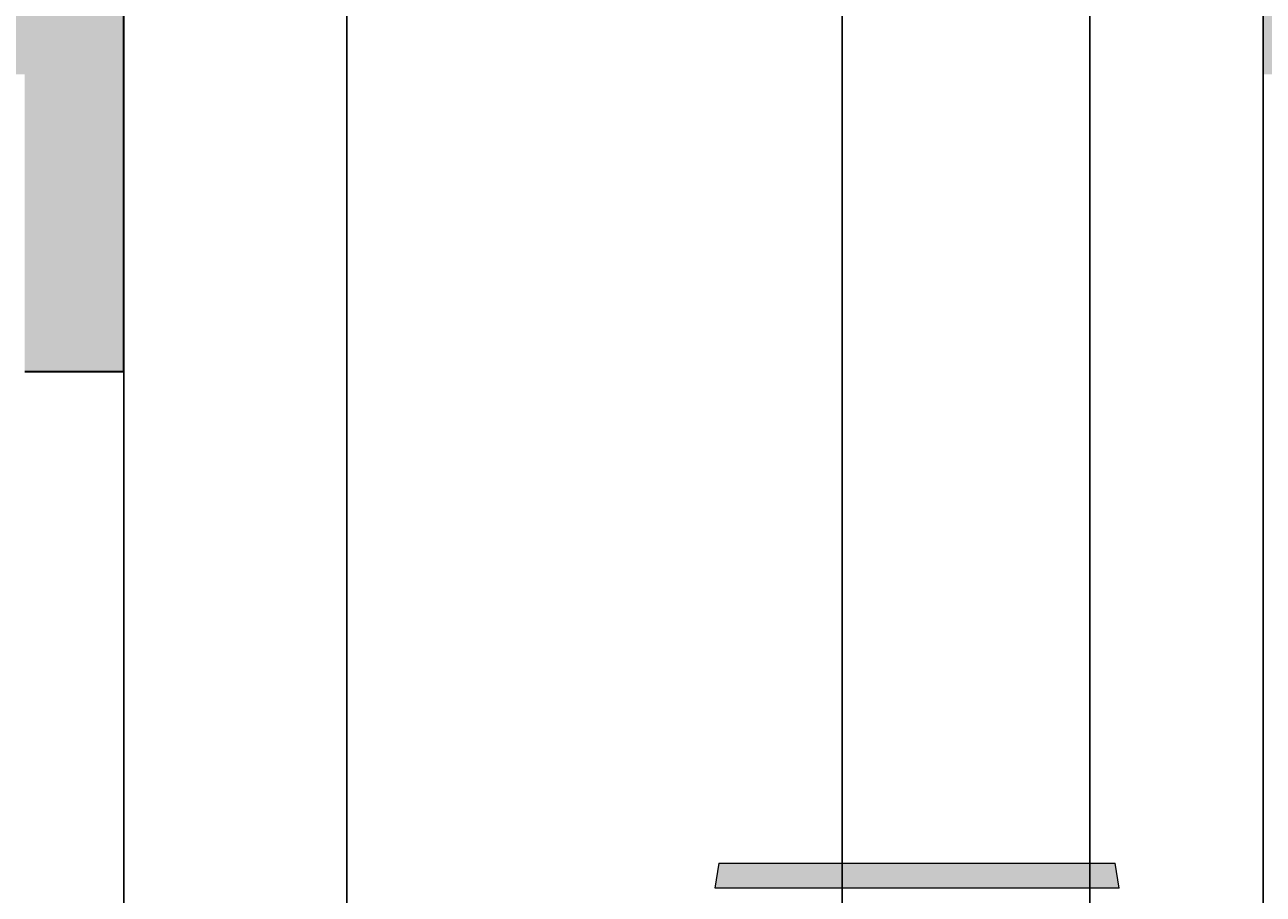
# Model space of a CAD drawing. Units: inches. Extents: x 1567 to 1964, y 1813 to 2447.
# Tile 18 of 28: x 1738 to 1788, y 2226 to 2261. Entities that reach past the tile are written whole.
import ezdxf

# ---------------------------------------------------------------- set-up
doc = ezdxf.new("R2010")
doc.units = ezdxf.units.IN
for name, color, linetype, lineweight in [('A-ANNO-DIMS', 2, 'Continuous', 18), ('A-FURN', 8, 'Continuous', 18), ('A-WALL', 7, 'Continuous', 35)]:
    doc.layers.add(name, color=color, linetype=linetype, lineweight=lineweight)
doc.layers.add('A-FURN-PATT', color=252, linetype='Continuous', lineweight=13, true_color=0x939598)
doc.layers.add('A-WALL-PATT', color=251, linetype='Continuous', lineweight=13, true_color=0x636466)
doc.styles.get("Standard").update_dxf_attribs({"font": 'arial.ttf'})
doc.dimstyles.get("Standard").update_dxf_attribs({"dimtxt": 0.18, "dimasz": 0.18, "dimexe": 0.18, "dimexo": 0.0625, "dimgap": 0.09, "dimtad": 0, "dimtih": 1, "dimtoh": 1, "dimdec": 4, "dimzin": 0, "dimdsep": 46, "dimtxsty": 'Standard', "dimcen": 0.09, "dimadec": 0, "dimazin": 0, "dimtfac": 1, "dimtdec": 4, "dimtofl": 0, "dimtmove": 0, "dimatfit": 3, "dimfxl": 1, "dimtolj": 1, "dimtzin": 0, "dimarcsym": 0})

# ---------------------------------------------------------------- blocks, each defined once
blk = doc.blocks.new('Dining Set - 36 x 72 in.')
for p, q in [((-22, 27.5), (-22.1562, 26.50042)), ((-22, 27.5), (-6, 27.5)), ((-5.8437, 26.49966), (-6, 27.5)), ((-5.8416, 26.5), (-22.1534, 26.5))]:
    blk.add_line(p, q)
blk = doc.blocks.new('*D47')
at = {"layer": 'A-ANNO-DIMS', "color": 0, "lineweight": -2, "transparency": 16777216}
for p, q in [((1742.43, 2331.227), (1742.43, 1813.46)), ((1788.43, 2331.227), (1788.43, 1813.46)), ((1742.61, 1813.64), (1765.207, 1813.64)), ((1788.25, 1813.64), (1765.652, 1813.64))]:
    blk.add_line(p, q, dxfattribs=at)
at = {"layer": 'A-ANNO-DIMS', "color": 0, "transparency": 16777216}
for points in [[(1742.61, 1813.67), (1742.61, 1813.61), (1742.43, 1813.64)], [(1788.25, 1813.67), (1788.25, 1813.61), (1788.43, 1813.64)]]:
    blk.add_solid(points, dxfattribs=at)
at = {"layer": 'Defpoints', "color": 0, "transparency": 16777216}
for p in [(1742.43, 2331.29), (1788.43, 2331.29), (1788.43, 1813.64)]:
    blk.add_point(p, dxfattribs=at)
at = {"layer": 'A-ANNO-DIMS', "color": 0, "transparency": 16777216, "insert": (1765.43, 1813.64), "char_height": 0.18, "attachment_point": 5}
blk.add_mtext('\\A1;46', dxfattribs=at)
blk = doc.blocks.new('*D54')
at = {"layer": 'A-ANNO-DIMS', "color": 0, "lineweight": -2, "transparency": 16777216}
for p, q in [((1711.43, 1964.352), (1711.43, 2447.12)), ((1795.43, 1964.352), (1795.43, 2447.12)), ((1711.61, 2446.94), (1753.211, 2446.94)), ((1795.25, 2446.94), (1753.648, 2446.94))]:
    blk.add_line(p, q, dxfattribs=at)
at = {"layer": 'A-ANNO-DIMS', "color": 0, "transparency": 16777216}
for points in [[(1711.61, 2446.97), (1711.61, 2446.91), (1711.43, 2446.94)], [(1795.25, 2446.97), (1795.25, 2446.91), (1795.43, 2446.94)]]:
    blk.add_solid(points, dxfattribs=at)
at = {"layer": 'Defpoints', "color": 0, "transparency": 16777216}
for p in [(1795.43, 2446.94), (1711.43, 1964.29), (1795.43, 1964.29)]:
    blk.add_point(p, dxfattribs=at)
at = {"layer": 'A-ANNO-DIMS', "color": 0, "transparency": 16777216, "insert": (1753.43, 2446.94), "char_height": 0.18, "attachment_point": 5}
blk.add_mtext('\\A1;84', dxfattribs=at)
blk = doc.blocks.new('*D58')
at = {"layer": 'A-ANNO-DIMS', "color": 0, "lineweight": -2, "transparency": 16777216}
for p, q in [((1742.43, 2127.352), (1742.43, 2447.12)), ((1751.43, 2127.352), (1751.43, 2447.12)), ((1742.61, 2446.94), (1746.78, 2446.94)), ((1751.25, 2446.94), (1747.079, 2446.94))]:
    blk.add_line(p, q, dxfattribs=at)
at = {"layer": 'A-ANNO-DIMS', "color": 0, "transparency": 16777216}
for points in [[(1742.61, 2446.97), (1742.61, 2446.91), (1742.43, 2446.94)], [(1751.25, 2446.97), (1751.25, 2446.91), (1751.43, 2446.94)]]:
    blk.add_solid(points, dxfattribs=at)
at = {"layer": 'Defpoints', "color": 0, "transparency": 16777216}
for p in [(1751.43, 2446.94), (1742.43, 2127.29), (1751.43, 2127.29)]:
    blk.add_point(p, dxfattribs=at)
at = {"layer": 'A-ANNO-DIMS', "color": 0, "transparency": 16777216, "insert": (1746.93, 2446.94), "char_height": 0.18, "attachment_point": 5}
blk.add_mtext('\\A1;9', dxfattribs=at)
blk = doc.blocks.new('*D59')
at = {"layer": 'A-ANNO-DIMS', "color": 0, "lineweight": -2, "transparency": 16777216}
for p, q in [((1751.43, 2127.352), (1751.43, 2447.12)), ((1781.43, 2127.352), (1781.43, 2447.12)), ((1751.61, 2446.94), (1766.211, 2446.94)), ((1781.25, 2446.94), (1766.648, 2446.94))]:
    blk.add_line(p, q, dxfattribs=at)
at = {"layer": 'A-ANNO-DIMS', "color": 0, "transparency": 16777216}
for points in [[(1751.61, 2446.97), (1751.61, 2446.91), (1751.43, 2446.94)], [(1781.25, 2446.97), (1781.25, 2446.91), (1781.43, 2446.94)]]:
    blk.add_solid(points, dxfattribs=at)
at = {"layer": 'Defpoints', "color": 0, "transparency": 16777216}
for p in [(1781.43, 2446.94), (1751.43, 2127.29), (1781.43, 2127.29)]:
    blk.add_point(p, dxfattribs=at)
at = {"layer": 'A-ANNO-DIMS', "color": 0, "transparency": 16777216, "insert": (1766.43, 2446.94), "char_height": 0.18, "attachment_point": 5}
blk.add_mtext('\\A1;30', dxfattribs=at)
blk = doc.blocks.new('*D63')
at = {"layer": 'A-ANNO-DIMS', "color": 0, "lineweight": -2, "transparency": 16777216}
for p, q in [((1735.43, 1988.352), (1735.43, 2447.12)), ((1771.43, 1988.352), (1771.43, 2447.12)), ((1735.61, 2446.94), (1753.211, 2446.94)), ((1771.25, 2446.94), (1753.648, 2446.94))]:
    blk.add_line(p, q, dxfattribs=at)
at = {"layer": 'A-ANNO-DIMS', "color": 0, "transparency": 16777216}
for points in [[(1735.61, 2446.97), (1735.61, 2446.91), (1735.43, 2446.94)], [(1771.25, 2446.97), (1771.25, 2446.91), (1771.43, 2446.94)]]:
    blk.add_solid(points, dxfattribs=at)
at = {"layer": 'Defpoints', "color": 0, "transparency": 16777216}
for p in [(1771.43, 2446.94), (1735.43, 1988.29), (1771.43, 1988.29)]:
    blk.add_point(p, dxfattribs=at)
at = {"layer": 'A-ANNO-DIMS', "color": 0, "transparency": 16777216, "insert": (1753.43, 2446.94), "char_height": 0.18, "attachment_point": 5}
blk.add_mtext('\\A1;36', dxfattribs=at)

msp = doc.modelspace()

# ---------------------------------------------------------------- hatches: boundary and pattern name
at = {"layer": 'A-FURN-PATT'}
h = msp.add_hatch(color=256, dxfattribs=at)
h.dxf.hatch_style = 1
h.paths.add_polyline_path([(1621.2532, 2242.0229), (1643.7811, 2241.7239), (1643.8607, 2247.7234), (1617.863, 2248.0685, 0.1904762), (1616.7481, 2164.0759), (1642.7458, 2163.7308), (1642.8254, 2169.7302), (1620.2975, 2170.0293, -0.1519478)])
h.paths.add_polyline_path([(1673.5306, 2249.6607), (1653.8509, 2249.6607), (1653.8509, 2248.5031, 0.1176471), (1673.5306, 2248.5031)])
h.paths.add_polyline_path([(1706.0889, 2249.6607), (1686.4092, 2249.6607), (1686.4092, 2248.5031, 0.1176471), (1706.0889, 2248.5031)])
h.paths.add_polyline_path([(1782.4511, 2227.4197), (1766.4511, 2227.4197), (1766.2949, 2226.4197), (1782.6074, 2226.4197)])
h.paths.add_polyline_path([(1810.4511, 2227.4197), (1794.4511, 2227.4197), (1794.2949, 2226.4197), (1810.6074, 2226.4197)])
h.paths.add_polyline_path([(1743.9511, 2208.076), (1742.9511, 2207.9197), (1742.9511, 2191.9197), (1743.9511, 2191.7635)])
h.paths.add_polyline_path([(1782.6074, 2173.4197), (1766.2949, 2173.4197), (1766.4511, 2172.4197), (1782.4511, 2172.4197)])
h.paths.add_polyline_path([(1810.6074, 2173.4197), (1794.2949, 2173.4197), (1794.4511, 2172.4197), (1810.4511, 2172.4197)])
h.paths.add_polyline_path([(1861.053, 2006.5071), (1845.8531, 2006.5071), (1861.053, 1991.3071)])
h.paths.add_polyline_path([(1905.853, 1993.7071), (1861.053, 1993.7071), (1861.053, 1991.3071), (1905.853, 1991.3071)])
h.paths.add_polyline_path([(1919.7245, 2257.29, 0.5000001), (1918.7245, 2258.29), (1901.7245, 2258.29, 0.5000001), (1900.7245, 2257.29), (1900.7245, 2253.29, 0.5000001), (1901.7245, 2252.29), (1918.7245, 2252.29, 0.5000001), (1919.7245, 2253.29)])
h.paths.add_polyline_path([(1875.9094, 2391.0204), (1875.9094, 2375.8204), (1891.1093, 2375.8204)], flags=17)
h.paths.add_polyline_path([(1891.1093, 2405.4204), (1831.1094, 2405.4204), (1831.1094, 2391.0204), (1839.1093, 2391.0204), (1839.1093, 2404.2204), (1859.9093, 2404.2204), (1859.9093, 2391.0204), (1862.3093, 2391.0204), (1862.3093, 2404.2204), (1883.1093, 2404.2204), (1883.1093, 2389.0204), (1877.9094, 2389.0204), (1891.1093, 2375.8204)])
h.paths.add_polyline_path([(1682.1402, 2390.0316), (1682.1402, 2374.8316), (1697.3402, 2374.8316)], flags=17)
h.paths.add_polyline_path([(1697.3402, 2404.4316), (1637.3402, 2404.4316), (1637.3402, 2390.0316), (1645.3402, 2390.0316), (1645.3402, 2403.2316), (1666.1402, 2403.2316), (1666.1402, 2390.0316), (1668.5402, 2390.0316), (1668.5402, 2403.2316), (1689.3402, 2403.2316), (1689.3402, 2388.0316), (1684.1402, 2388.0316), (1697.3402, 2374.8316)])
at = {"layer": 'A-WALL-PATT'}
h = msp.add_hatch(color=256, dxfattribs=at)
h.dxf.hatch_style = 1
h.paths.add_polyline_path([(1606.4295, 2407.29), (1654.4295, 2407.29), (1654.4295, 2416.29), (1597.4295, 2416.29), (1597.4295, 2217.29), (1606.4295, 2217.29), (1606.4295, 2259.29), (1738.4295, 2259.29), (1738.4295, 2247.29), (1742.4295, 2247.29), (1742.4295, 2259.29), (1742.4295, 2272.29), (1738.4295, 2272.29), (1738.4295, 2263.29), (1606.4295, 2263.29)])
h.paths.add_polyline_path([(1753.4295, 2416.29), (1690.4295, 2416.29), (1690.4295, 2407.29), (1738.4295, 2407.29), (1738.4295, 2308.29), (1742.4295, 2308.29), (1742.4295, 2331.29), (1746.9295, 2331.29), (1746.9295, 2335.29), (1742.4295, 2335.29), (1742.4295, 2407.29), (1753.4295, 2407.29)])
h.paths.add_polyline_path([(1840.4295, 2416.29), (1777.4295, 2416.29), (1777.4295, 2407.29), (1788.4295, 2407.29), (1788.4295, 2335.29), (1776.9295, 2335.29), (1776.9295, 2331.29), (1788.4295, 2331.29), (1788.4295, 2308.29), (1792.4295, 2308.29), (1792.4295, 2407.29), (1840.4295, 2407.29)])
h.paths.add_polyline_path([(1933.4295, 2416.29), (1876.4295, 2416.29), (1876.4295, 2407.29), (1924.4295, 2407.29), (1924.4295, 2263.29), (1792.4295, 2263.29), (1792.4295, 2272.29), (1788.4295, 2272.29), (1788.4295, 2259.29), (1872.4295, 2259.29), (1872.4295, 2171.29), (1880.9295, 2171.29), (1880.9295, 2175.29), (1876.4295, 2175.29), (1876.4295, 2259.29), (1924.4295, 2259.29), (1924.4295, 2229.29), (1933.4295, 2229.29)])
h.paths.add_polyline_path([(1933.4295, 2205.29), (1924.4295, 2205.29), (1924.4295, 2175.29), (1910.9295, 2175.29), (1910.9295, 2171.29), (1924.4295, 2171.29), (1924.4295, 2127.29), (1844.4295, 2127.29), (1844.4295, 2123.29), (1924.4295, 2123.29), (1924.4295, 2063.29), (1933.4295, 2063.29)])
h.paths.add_polyline_path([(1799.4295, 2123.29), (1808.4295, 2123.29), (1808.4295, 2127.29), (1781.4295, 2127.29), (1781.4295, 2123.29), (1795.4295, 2123.29), (1795.4295, 1964.29), (1711.4295, 1964.29), (1711.4295, 2123.29), (1751.4295, 2123.29), (1751.4295, 2127.29), (1742.4295, 2127.29), (1742.4295, 2139.29), (1738.4295, 2139.29), (1738.4295, 2127.29), (1678.4295, 2127.29), (1678.4295, 2123.29), (1702.4295, 2123.29), (1702.4295, 1913.29), (1678.4295, 1913.29), (1678.4295, 1904.29), (1711.4295, 1904.29), (1711.4295, 1960.29), (1795.4295, 1960.29), (1795.4295, 1906.69), (1929.4295, 1906.69), (1929.4295, 1848.29), (1601.4295, 1848.29), (1601.4295, 1904.29), (1630.4295, 1904.29), (1630.4295, 1913.29), (1606.4295, 1913.29), (1606.4295, 2123.29), (1630.4295, 2123.29), (1630.4295, 2127.29), (1606.4295, 2127.29), (1606.4295, 2169.29), (1597.4295, 2169.29), (1597.4295, 1844.29), (1933.4295, 1844.29), (1933.4295, 2027.29), (1924.4295, 2027.29), (1924.4295, 1967.29), (1833.9295, 1967.29), (1833.9295, 1963.29), (1924.4295, 1963.29), (1924.4295, 1910.69), (1799.4295, 1910.69), (1799.4295, 1963.29), (1803.9295, 1963.29), (1803.9295, 1967.29), (1799.4295, 1967.29)])

# ---------------------------------------------------------------- linework, layer by layer
at = {"layer": 'A-WALL'}
for p, q in [((1742.4295, 2259.29), (1742.4295, 2272.29)), ((1742.4295, 2247.29), (1742.4295, 2259.29)), ((1738.4295, 2247.29), (1742.4295, 2247.29))]:
    msp.add_line(p, q, dxfattribs=at)

# ---------------------------------------------------------------- block references
at = {"layer": 'A-FURN'}
msp.add_blockref('Dining Set - 36 x 72 in.', (1788.4511, 2199.9197), dxfattribs=at)

# ---------------------------------------------------------------- dimensions: what is measured, and where the dimension line sits
at = {"layer": 'A-ANNO-DIMS'}
for base, p1, p2, picture, middle in [((1795.4295, 2446.94), (1711.4295, 1964.29), (1795.4295, 1964.29), '*D54', (1753.4295, 2446.94)), ((1771.4295, 2446.94), (1735.4295, 1988.29), (1771.4295, 1988.29), '*D63', (1753.4295, 2446.94)), ((1751.4295, 2446.94), (1742.4295, 2127.29), (1751.4295, 2127.29), '*D58', (1746.9295, 2446.94)), ((1781.4295, 2446.94), (1751.4295, 2127.29), (1781.4295, 2127.29), '*D59', (1766.4295, 2446.94)), ((1788.4295, 1813.64), (1742.4295, 2331.29), (1788.4295, 2331.29), '*D47', (1765.4295, 1813.64))]:
    dim = msp.add_linear_dim(base=base, p1=p1, p2=p2, dimstyle='Standard', override={"dimdec": 0, "dimlfac": 1, "dimrnd": 0, "dimzin": 0, "dimdsep": 46, "dimlunit": 2}, dxfattribs=at)
    dim.commit()
    dim.dimension.update_dxf_attribs({"geometry": picture, "text_midpoint": middle})

doc.saveas('drawing.dxf')
